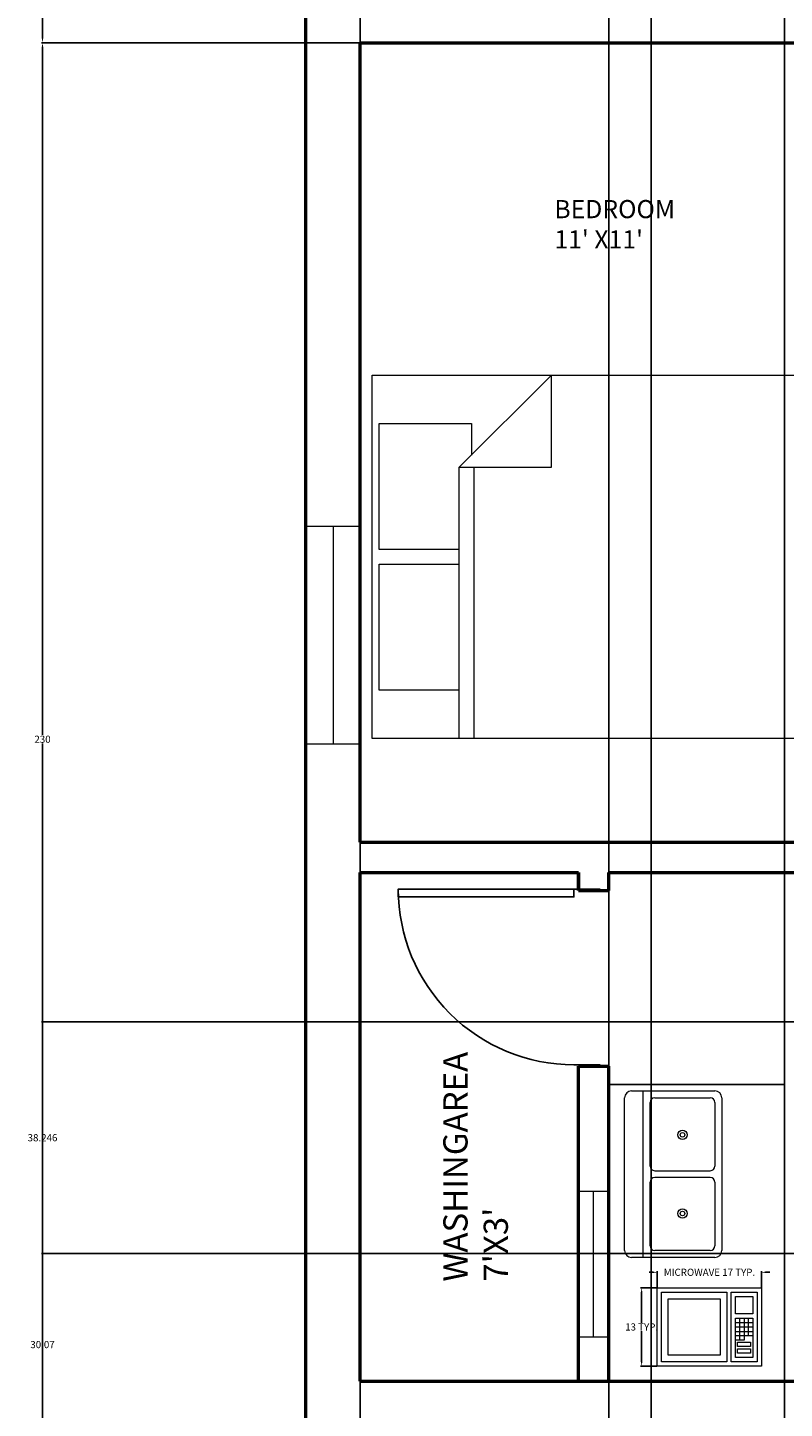
# Model space of a CAD drawing. Units: inches. Extents: x 3506 to 3958, y 1553 to 2506.
# Tile 3 of 16: x 3506 to 3631, y 1775 to 2003. Entities that reach past the tile are written whole.
import ezdxf

# ---------------------------------------------------------------- set-up
doc = ezdxf.new("R2010")
doc.units = ezdxf.units.IN
doc.header["$MEASUREMENT"] = 0
for name, color, linetype, lineweight in [('A-ANNO-DIMS', 2, 'Continuous', 18), ('A-AREA-IDEN', 7, 'Continuous', 18), ('A-FLOR-CASE', 7, 'Continuous', 25), ('A-WALL', 7, 'Continuous', 50), ('doors', 40, 'Continuous', 25), ('furniture', 120, 'Continuous', 18), ('kitchen', 181, 'Continuous', 18), ('window', 30, 'Continuous', 20)]:
    doc.layers.add(name, color=color, linetype=linetype, lineweight=lineweight)
doc.layers.add('A-WALL-PATT', color=251, linetype='Continuous', lineweight=13, true_color=0x636466)
doc.styles.get("Standard").update_dxf_attribs({"font": 'arial.ttf'})
doc.dimstyles.get("Standard").update_dxf_attribs({"dimtxt": 1.18, "dimasz": 0.68, "dimexe": 0.18, "dimexo": 0.0625, "dimgap": 0.09, "dimtad": 0, "dimtih": 1, "dimtoh": 1, "dimdec": 1, "dimzin": 0, "dimdsep": 46, "dimlunit": 3, "dimtxsty": 'Standard', "dimcen": 0.09, "dimadec": 0, "dimazin": 0, "dimtfac": 1, "dimtdec": 1, "dimtofl": 0, "dimtmove": 0, "dimatfit": 3, "dimfxl": 1, "dimtolj": 1, "dimtzin": 0, "dimarcsym": 0})

# ---------------------------------------------------------------- blocks, each defined once
blk = doc.blocks.new('*U12')
for p, q in [((0, 0), (0, 6)), ((40, 0), (40, 6))]:
    blk.add_line(p, q)
blk.add_lwpolyline([(0, 0), (0, -40), (1.75, -40), (1.75, 0)], close=True)
blk.add_arc((0, 0), 40, 270, 0)
blk = doc.blocks.new('Bed - Queen')
for p, q in [((0, -80.00003), (0, 0)), ((0, 0), (59.99999, 0)), ((59.99999, 0), (59.99999, -80.00003)), ((7.99999, -1.2), (28.79998, -1.2)), ((7.99999, -14.4), (7.99999, -1.2)), ((28.79998, -1.2), (28.79998, -14.4)), ((31.19999, -1.2), (51.99999, -1.2)), ((31.19999, -14.4), (31.19999, -1.2)), ((51.99999, -1.2), (51.99999, -16.4)), ((0, -14.4), (44.8, -14.4)), ((59.99999, -29.6), (44.8, -14.4)), ((44.8, -14.4), (44.8, -29.6)), ((44.8, -16.8), (0, -16.8)), ((51.99999, -16.4), (46.79936, -16.4)), ((44.8, -29.6), (59.99999, -29.6)), ((59.99999, -80.00003), (0, -80.00003))]:
    blk.add_line(p, q)
blk = doc.blocks.new('Microwave')
for p, q in [((18, 10), (22, 10)), ((19, 7), (19, 11)), ((20, 11), (20, 7)), ((21, 7), (21, 11)), ((22, 9), (18, 9)), ((18, 8), (22, 8)), ((22, 7), (18, 7)), ((19, 6), (19, 7)), ((20, 7), (20, 6)), ((20, 6), (18, 6))]:
    blk.add_line(p, q)
for points in [[(0, 0), (0, 18), (24, 18), (24, 0)], [(1, 1), (1, 17), (16, 17), (16, 1)], [(17, 1), (17, 17), (23, 17), (23, 1)], [(18, 12), (18, 16), (22, 16), (22, 12)], [(2.5, 2.5), (2.5, 15.5), (14.5, 15.5), (14.5, 2.5)], [(18, 2), (18, 11), (22, 11), (22, 2)], [(18.5, 4.5), (18.5, 5.5), (21.5, 5.5), (21.5, 4.5)], [(18.5, 3), (18.5, 4), (21.5, 4), (21.5, 3)]]:
    blk.add_lwpolyline(points, close=True)
blk = doc.blocks.new('Sink-double - 36 in top')
for p, q in [((-18, -4), (18, -4)), ((-0.75, -18.5), (-0.75, -6.5)), ((0.75, -6.5), (0.75, -18.5))]:
    blk.add_line(p, q)
for points in [[(-16.5, 0), (16.5, 0)], [(-18, -19.5), (-18, -1.5)], [(18, -1.5), (18, -19.5)], [(-15.5, -5.5), (-1.75, -5.5)], [(1.75, -5.5), (15.5, -5.5)], [(-16.5, -18.5), (-16.5, -6.5)], [(16.5, -6.5), (16.5, -18.5)], [(-1.75, -19.5), (-15.5, -19.5)], [(15.5, -19.5), (1.75, -19.5)], [(16.5, -21), (-16.5, -21)]]:
    blk.add_lwpolyline(points)
for centre, radius in [((-8.5, -12.5), 1), ((8.5, -12.5), 1), ((-8.5, -12.5), 0.5), ((8.5, -12.5), 0.5)]:
    blk.add_circle(centre, radius)
for centre, radius, start, end in [((-16.5, -1.5), 1.5, 90, 180), ((16.5, -1.5), 1.5, 0, 90), ((-15.5, -6.5), 1, 90, 180), ((-1.75, -6.5), 1, 0, 90), ((1.75, -6.5), 1, 90, 180), ((15.5, -6.5), 1, 0, 90), ((-16.5, -19.5), 1.5, 180, 270), ((-15.5, -18.5), 1, 180, 270), ((-1.75, -18.5), 1, 270, 0), ((1.75, -18.5), 1, 180, 270), ((15.5, -18.5), 1, 270, 0), ((16.5, -19.5), 1.5, 270, 0)]:
    blk.add_arc(centre, radius, start, end)
blk = doc.blocks.new('WIN-36IN-9IN-WALL')
for p, q in [((0, 9), (0, 0)), ((36, 9), (0, 9)), ((0, 9), (0, 4.5)), ((36, 0), (36, 9)), ((0, 4.5), (36, 4.5)), ((0, 0), (36, 0))]:
    blk.add_line(p, q)
blk = doc.blocks.new('WIN-24IN-5IN-PARTITION')
for p, q in [((5, 24), (0, 24)), ((0, 24), (0, 0)), ((2.5, 0), (2.5, 24)), ((5, 0), (5, 24)), ((0, 0), (5, 0)), ((0, 0), (2.5, 0))]:
    blk.add_line(p, q)
blk = doc.blocks.new('*D20')
at = {"layer": 'A-ANNO-DIMS', "color": 0, "lineweight": -2, "transparency": 16777216}
for p, q in [((3609.07, 1797.37), (3608.39, 1797.37)), ((3609.75, 1794.85), (3609.75, 1797.55)), ((3626.96, 1794.85), (3626.96, 1797.55)), ((3627.64, 1797.37), (3628.32, 1797.37))]:
    blk.add_line(p, q, dxfattribs=at)
at = {"layer": 'A-ANNO-DIMS', "color": 0, "transparency": 16777216}
for points in [[(3609.07, 1797.48), (3609.07, 1797.25), (3609.75, 1797.37)], [(3627.64, 1797.48), (3627.64, 1797.25), (3626.96, 1797.37)]]:
    blk.add_solid(points, dxfattribs=at)
at = {"layer": 'Defpoints', "color": 0, "transparency": 16777216}
for p in [(3626.96, 1797.37), (3609.75, 1794.79), (3626.96, 1794.79)]:
    blk.add_point(p, dxfattribs=at)
at = {"layer": 'A-ANNO-DIMS', "color": 0, "transparency": 16777216, "insert": (3618.36, 1797.37), "char_height": 1.18, "attachment_point": 5}
blk.add_mtext('\\A1;MICROWAVE 17 TYP.', dxfattribs=at)
blk = doc.blocks.new('*D21')
at = {"layer": 'A-ANNO-DIMS', "color": 0, "lineweight": -2, "transparency": 16777216}
for p, q in [((3609.69, 1794.79), (3606.99, 1794.79)), ((3607.17, 1794.11), (3607.17, 1789.03)), ((3607.17, 1782.56), (3607.17, 1787.64)), ((3609.69, 1781.88), (3606.99, 1781.88))]:
    blk.add_line(p, q, dxfattribs=at)
at = {"layer": 'A-ANNO-DIMS', "color": 0, "transparency": 16777216}
for points in [[(3607.06, 1794.11), (3607.29, 1794.11), (3607.17, 1794.79)], [(3607.06, 1782.56), (3607.29, 1782.56), (3607.17, 1781.88)]]:
    blk.add_solid(points, dxfattribs=at)
at = {"layer": 'Defpoints', "color": 0, "transparency": 16777216}
for p in [(3607.17, 1794.79), (3609.75, 1794.79), (3609.75, 1781.88)]:
    blk.add_point(p, dxfattribs=at)
at = {"layer": 'A-ANNO-DIMS', "color": 0, "transparency": 16777216, "insert": (3607.17, 1788.34), "char_height": 1.18, "attachment_point": 5}
blk.add_mtext('\\A1;13 TYP.', dxfattribs=at)
blk = doc.blocks.new('*D42')
at = {"layer": 'A-ANNO-DIMS', "color": 0, "lineweight": -2, "transparency": 16777216}
for p, q in [((3560.67, 2000.39), (3508.1, 2000.39)), ((3508.28, 1999.71), (3508.28, 1886.09)), ((3508.28, 1771.07), (3508.28, 1884.7)), ((3560.67, 1770.39), (3508.1, 1770.39))]:
    blk.add_line(p, q, dxfattribs=at)
at = {"layer": 'A-ANNO-DIMS', "color": 0, "transparency": 16777216}
for points in [[(3508.17, 1999.71), (3508.39, 1999.71), (3508.28, 2000.39)], [(3508.17, 1771.07), (3508.39, 1771.07), (3508.28, 1770.39)]]:
    blk.add_solid(points, dxfattribs=at)
at = {"layer": 'Defpoints', "color": 0, "transparency": 16777216}
for p in [(3508.28, 2000.39), (3560.73, 2000.39), (3560.73, 1770.39)]:
    blk.add_point(p, dxfattribs=at)
at = {"layer": 'A-ANNO-DIMS', "color": 0, "transparency": 16777216, "insert": (3508.28, 1885.39), "char_height": 1.18, "attachment_point": 5}
blk.add_mtext('\\A1;230', dxfattribs=at)
blk = doc.blocks.new('*D43')
at = {"layer": 'A-ANNO-DIMS', "color": 0, "lineweight": -2, "transparency": 16777216}
for p, q in [((3560.67, 2226.39), (3508.1, 2226.39)), ((3508.28, 2225.71), (3508.28, 2114.09)), ((3508.28, 2001.07), (3508.28, 2112.7)), ((3560.67, 2000.39), (3508.1, 2000.39))]:
    blk.add_line(p, q, dxfattribs=at)
at = {"layer": 'A-ANNO-DIMS', "color": 0, "transparency": 16777216}
for points in [[(3508.17, 2225.71), (3508.39, 2225.71), (3508.28, 2226.39)], [(3508.17, 2001.07), (3508.39, 2001.07), (3508.28, 2000.39)]]:
    blk.add_solid(points, dxfattribs=at)
at = {"layer": 'Defpoints', "color": 0, "transparency": 16777216}
for p in [(3508.28, 2226.39), (3560.73, 2226.39), (3560.73, 2000.39)]:
    blk.add_point(p, dxfattribs=at)
at = {"layer": 'A-ANNO-DIMS', "color": 0, "transparency": 16777216, "insert": (3508.28, 2113.39), "char_height": 1.18, "attachment_point": 5}
blk.add_mtext('\\A1;226', dxfattribs=at)
blk = doc.blocks.new('*D50')
at = {"layer": 'A-ANNO-DIMS', "color": 0, "lineweight": -2, "transparency": 16777216}
for p, q in [((3608.73, 1606.46), (3608.73, 2505.02)), ((3609.41, 2504.84), (3672.39, 2504.84)), ((3738.05, 2504.84), (3675.07, 2504.84)), ((3738.73, 1606.46), (3738.73, 2505.02))]:
    blk.add_line(p, q, dxfattribs=at)
at = {"layer": 'A-ANNO-DIMS', "color": 0, "transparency": 16777216}
for points in [[(3609.41, 2504.96), (3609.41, 2504.73), (3608.73, 2504.84)], [(3738.05, 2504.96), (3738.05, 2504.73), (3738.73, 2504.84)]]:
    blk.add_solid(points, dxfattribs=at)
at = {"layer": 'Defpoints', "color": 0, "transparency": 16777216}
for p in [(3738.73, 2504.84), (3608.73, 1606.39), (3738.73, 1606.39)]:
    blk.add_point(p, dxfattribs=at)
at = {"layer": 'A-ANNO-DIMS', "color": 0, "transparency": 16777216, "insert": (3673.73, 2504.84), "char_height": 1.18, "attachment_point": 5}
blk.add_mtext('\\A1;130', dxfattribs=at)
blk = doc.blocks.new('*D52')
at = {"layer": 'A-ANNO-DIMS', "color": 0, "lineweight": -2, "transparency": 16777216}
for p, q in [((3560.73, 1606.46), (3560.73, 2505.02)), ((3561.41, 2504.84), (3583.77, 2504.84)), ((3608.05, 2504.84), (3585.69, 2504.84)), ((3608.73, 1606.46), (3608.73, 2505.02))]:
    blk.add_line(p, q, dxfattribs=at)
at = {"layer": 'A-ANNO-DIMS', "color": 0, "transparency": 16777216}
for points in [[(3561.41, 2504.96), (3561.41, 2504.73), (3560.73, 2504.84)], [(3608.05, 2504.96), (3608.05, 2504.73), (3608.73, 2504.84)]]:
    blk.add_solid(points, dxfattribs=at)
at = {"layer": 'Defpoints', "color": 0, "transparency": 16777216}
for p in [(3608.73, 2504.84), (3560.73, 1606.39), (3608.73, 1606.39)]:
    blk.add_point(p, dxfattribs=at)
at = {"layer": 'A-ANNO-DIMS', "color": 0, "transparency": 16777216, "insert": (3584.73, 2504.84), "char_height": 1.18, "attachment_point": 5}
blk.add_mtext('\\A1;48', dxfattribs=at)
blk = doc.blocks.new('*D62')
at = {"layer": 'A-ANNO-DIMS', "color": 0, "lineweight": -2, "transparency": 16777216}
for p, q in [((3860.67, 1838.71), (3508.1, 1838.71)), ((3508.28, 1838.03), (3508.28, 1820.28)), ((3508.28, 1801.14), (3508.28, 1818.89)), ((3860.67, 1800.46), (3508.1, 1800.46))]:
    blk.add_line(p, q, dxfattribs=at)
at = {"layer": 'A-ANNO-DIMS', "color": 0, "transparency": 16777216}
for points in [[(3508.17, 1838.03), (3508.39, 1838.03), (3508.28, 1838.71)], [(3508.17, 1801.14), (3508.39, 1801.14), (3508.28, 1800.46)]]:
    blk.add_solid(points, dxfattribs=at)
at = {"layer": 'Defpoints', "color": 0, "transparency": 16777216}
for p in [(3860.73, 1838.71), (3508.28, 1800.46), (3860.73, 1800.46)]:
    blk.add_point(p, dxfattribs=at)
at = {"layer": 'A-ANNO-DIMS', "color": 0, "transparency": 16777216, "insert": (3508.28, 1819.59), "char_height": 1.18, "attachment_point": 5}
blk.add_mtext('\\A1;38.246', dxfattribs=at)
blk = doc.blocks.new('*D63')
at = {"layer": 'A-ANNO-DIMS', "color": 0, "lineweight": -2, "transparency": 16777216}
for p, q in [((3869.67, 1800.46), (3508.1, 1800.46)), ((3508.28, 1799.78), (3508.28, 1786.12)), ((3508.28, 1771.07), (3508.28, 1784.74)), ((3869.67, 1770.39), (3508.1, 1770.39))]:
    blk.add_line(p, q, dxfattribs=at)
at = {"layer": 'A-ANNO-DIMS', "color": 0, "transparency": 16777216}
for points in [[(3508.17, 1799.78), (3508.39, 1799.78), (3508.28, 1800.46)], [(3508.17, 1771.07), (3508.39, 1771.07), (3508.28, 1770.39)]]:
    blk.add_solid(points, dxfattribs=at)
at = {"layer": 'Defpoints', "color": 0, "transparency": 16777216}
for p in [(3869.73, 1800.46), (3508.28, 1770.39), (3869.73, 1770.39)]:
    blk.add_point(p, dxfattribs=at)
at = {"layer": 'A-ANNO-DIMS', "color": 0, "transparency": 16777216, "insert": (3508.28, 1785.43), "char_height": 1.18, "attachment_point": 5}
blk.add_mtext('\\A1;30.07', dxfattribs=at)
blk = doc.blocks.new('*D68')
at = {"layer": 'A-ANNO-DIMS', "color": 0, "lineweight": -2, "transparency": 16777216}
for p, q in [((3630.73, 2260.33), (3630.73, 1553.76)), ((3601.73, 2231.33), (3601.73, 1553.76)), ((3602.41, 1553.94), (3615.28, 1553.94)), ((3630.05, 1553.94), (3617.18, 1553.94))]:
    blk.add_line(p, q, dxfattribs=at)
at = {"layer": 'A-ANNO-DIMS', "color": 0, "transparency": 16777216}
for points in [[(3602.41, 1554.06), (3602.41, 1553.83), (3601.73, 1553.94)], [(3630.05, 1554.06), (3630.05, 1553.83), (3630.73, 1553.94)]]:
    blk.add_solid(points, dxfattribs=at)
at = {"layer": 'Defpoints', "color": 0, "transparency": 16777216}
for p in [(3630.73, 2260.39), (3601.73, 2231.39), (3630.73, 1553.94)]:
    blk.add_point(p, dxfattribs=at)
at = {"layer": 'A-ANNO-DIMS', "color": 0, "transparency": 16777216, "insert": (3616.23, 1553.94), "char_height": 1.18, "attachment_point": 5}
blk.add_mtext('\\A1;29', dxfattribs=at)

msp = doc.modelspace()

# ---------------------------------------------------------------- hatches: boundary and pattern name
at = {"layer": 'A-WALL-PATT'}
h = msp.add_hatch(dxfattribs=at)
h.set_pattern_fill('ANSI31', color=256)
h.paths.add_polyline_path([(3911.7302, 2461.3942), (3551.7302, 2461.3942), (3551.7302, 2152.516), (3560.7302, 2152.516), (3560.7302, 2116.516), (3551.7302, 2116.516), (3551.7302, 1920.5711), (3556.2302, 1920.5711), (3560.7302, 1920.5711), (3560.7302, 2000.3942), (3692.7302, 2000.3942), (3692.7302, 1997.3942), (3697.7302, 1997.3942), (3697.7302, 2000.3942), (3771.7302, 2000.3942), (3771.7302, 1997.3942), (3776.7302, 1997.3942), (3776.7302, 1997.7206), (3778.5802, 1997.7206), (3807.5802, 1997.7206), (3807.5802, 1996.4519), (3778.5802, 1996.4519), (3778.5802, 1997.7206), (3776.7302, 1997.7206), (3776.7302, 1997.3942), (3771.7302, 1997.3942), (3771.7302, 2000.3942), (3697.7302, 2000.3942), (3697.7302, 1997.3942), (3692.7302, 1997.3942), (3689.8302, 1997.3942), (3689.8302, 1995.8192), (3653.8302, 1995.8192), (3653.8302, 1997.3942), (3689.8302, 1997.3942), (3692.7302, 1997.3942), (3692.7302, 2000.3942), (3560.7302, 2000.3942), (3560.7302, 1920.5711), (3551.7302, 1920.5711), (3551.7302, 1884.5711), (3551.7302, 1597.3942), (3911.7302, 1597.3942)], flags=17)
h.paths.add_polyline_path([(3596.7302, 2005.3942), (3596.7302, 2057.3035, -0.38730371), (3569.1778, 2085), (3569.15, 2085), (3569.15, 2086.2688), (3598.15, 2086.2688), (3598.15, 2085), (3569.1778, 2085, 0.38730371), (3596.7302, 2057.3035), (3596.7302, 2057.3942), (3601.7302, 2057.3942), (3601.7302, 2055.3942), (3630.7302, 2055.3942), (3630.7302, 2034.3942), (3694.7302, 2034.3942), (3694.7302, 2053.3942), (3699.7302, 2053.3942), (3699.7302, 2005.3942), (3860.7302, 2005.3942), (3860.7302, 2173.3942), (3771.7302, 2173.3942), (3771.7302, 2194.3942), (3776.7302, 2194.3942), (3776.7302, 2178.3942), (3860.7302, 2178.3942), (3860.7302, 2231.3942), (3601.7302, 2231.3942), (3601.7302, 2241.426), (3596.7302, 2241.426), (3596.7302, 2231.3942), (3560.7302, 2231.3942), (3560.7302, 2315.3942), (3596.7302, 2315.3942), (3596.7302, 2312.3942), (3601.7302, 2312.3942), (3601.7302, 2315.3942), (3697.7302, 2315.3942), (3697.7302, 2413.3942), (3692.7302, 2413.3942), (3692.7302, 2320.3942), (3560.7302, 2320.3942), (3560.7302, 2452.3942), (3692.7302, 2452.3942), (3692.7302, 2449.3942), (3697.7302, 2449.3942), (3697.7302, 2452.3942), (3771.7302, 2452.3942), (3771.7302, 2449.3942), (3776.7302, 2449.3942), (3776.7302, 2452.3942), (3860.7302, 2452.3942), (3860.7302, 2437.2075), (3865.2302, 2437.2075), (3865.2302, 2413.2075), (3860.7302, 2413.2075), (3860.7302, 2367.6976), (3865.2302, 2367.6976), (3869.7302, 2367.6976), (3869.7302, 2319.6976), (3860.7302, 2319.6976), (3860.7302, 2211.6248), (3869.7302, 2211.6248), (3869.7302, 2187.6248), (3860.7302, 2187.6248), (3860.7302, 2138.4346), (3865.2302, 2138.4346), (3869.7302, 2138.4346), (3869.7302, 2090.4346), (3860.7302, 2090.4346), (3860.7302, 1985.8449), (3869.7302, 1985.8449), (3869.7302, 1961.8449), (3860.7302, 1961.8449), (3860.7302, 1897.0756), (3865.2302, 1897.0756), (3869.7302, 1897.0756), (3869.7302, 1849.0756), (3860.7302, 1849.0756), (3860.7302, 1847.8112), (3860.7302, 1779.3942), (3596.7302, 1779.3942), (3596.7302, 1831.3942), (3601.7302, 1831.3942), (3601.7302, 1828.3942), (3630.7302, 1828.3942), (3630.7302, 1808.3942), (3691.7302, 1808.3942), (3691.7302, 1815.3942), (3696.7302, 1815.3942), (3696.7302, 1779.3942), (3860.7302, 1779.3942), (3860.7302, 1947.3942), (3771.7302, 1947.3942), (3771.7302, 1968.3942), (3776.7302, 1968.3942), (3776.7302, 1952.3942), (3860.7302, 1952.3942), (3860.7302, 2005.3942)], flags=0)
h.paths.add_polyline_path([(3596.7302, 2038.8546), (3601.7302, 2038.8546), (3601.7302, 2014.8546), (3596.7302, 2014.8546)], flags=0)
h.paths.add_polyline_path([(3564.1688, 2107), (3564.1688, 2167), (3644.1688, 2167), (3644.1688, 2107)], flags=0)
h.paths.add_polyline_path([(3607.0972, 2052.0208), (3620.8472, 2052.0208, -0.41421356), (3621.9931, 2050.875), (3621.9931, 2025.6667, -0.41421356), (3620.8472, 2024.5208), (3607.0972, 2024.5208, -0.41421356), (3605.9514, 2025.6667), (3605.9514, 2050.875, -0.41421356)], flags=0)
h.paths.add_polyline_path([(3578.5688, 2115), (3565.3688, 2115), (3565.3688, 2135.8), (3578.5688, 2135.8), (3578.5688, 2138.2), (3565.3688, 2138.2), (3565.3688, 2159), (3580.5688, 2159), (3580.5688, 2153.8), (3593.7688, 2167), (3593.7688, 2151.8), (3578.5688, 2151.8)], flags=0)
h.paths.add_polyline_path([(3610.9167, 2050.875), (3620.0833, 2050.875, -0.41421356), (3620.8472, 2050.1111), (3620.8472, 2039.6076, -0.41421356), (3620.0833, 2038.8438), (3610.9167, 2038.8438, -0.41421356), (3610.1528, 2039.6076), (3610.1528, 2050.1111, -0.41421356)], flags=0)
h.paths.add_polyline_path([(3610.9167, 2037.6979), (3620.0833, 2037.6979, -0.41421356), (3620.8472, 2036.934), (3620.8472, 2026.4306, -0.41421356), (3620.0833, 2025.6667), (3610.9167, 2025.6667, -0.41421356), (3610.1528, 2026.4306), (3610.1528, 2036.934, -0.41421356)], flags=0)
h.paths.add_polyline_path([(3616.2639, 2044.7639, -1), (3614.7361, 2044.7639, -1)], flags=0)
h.paths.add_polyline_path([(3615.8819, 2044.7639, -1), (3615.1181, 2044.7639, -1)], flags=0)
h.paths.add_polyline_path([(3616.2639, 2031.7778, -1), (3614.7361, 2031.7778, -1)], flags=0)
h.paths.add_polyline_path([(3615.8819, 2031.7778, -1), (3615.1181, 2031.7778, -1)], flags=0)
h.paths.add_polyline_path([(3609.7539, 2021.7868), (3626.9586, 2021.7868), (3626.9586, 2008.8833), (3609.7539, 2008.8833)], flags=0)
h.paths.add_polyline_path([(3610.4708, 2021.07), (3621.2237, 2021.07), (3621.2237, 2009.6002), (3610.4708, 2009.6002)], flags=0)
h.paths.add_polyline_path([(3611.5461, 2019.9947), (3620.1484, 2019.9947), (3620.1484, 2010.6755), (3611.5461, 2010.6755)], flags=0)
h.paths.add_polyline_path([(3621.9405, 2021.07), (3626.2417, 2021.07), (3626.2417, 2009.6002), (3621.9405, 2009.6002)], flags=0)
h.paths.add_polyline_path([(3622.6574, 2020.3531), (3625.5248, 2020.3531), (3625.5248, 2017.4857), (3622.6574, 2017.4857)], flags=0)
h.paths.add_polyline_path([(3622.6574, 2016.7688), (3625.5248, 2016.7688), (3625.5248, 2010.317), (3622.6574, 2010.317)], flags=0)
h.paths.add_polyline_path([(3624.808, 2016.0519), (3624.808, 2013.9013), (3624.0911, 2013.9013), (3624.0911, 2013.1845), (3623.3743, 2013.1845), (3623.3743, 2013.9013), (3623.3743, 2016.0519)], flags=0)
h.paths.add_polyline_path([(3623.0158, 2012.8261), (3625.1664, 2012.8261), (3625.1664, 2012.1092), (3623.0158, 2012.1092)], flags=0)
h.paths.add_polyline_path([(3623.0158, 2011.7508), (3625.1664, 2011.7508), (3625.1664, 2011.0339), (3623.0158, 2011.0339)], flags=0)
h.paths.add_polyline_path([(3650.0591, 2031.8202), (3674.0368, 2031.8202), (3674.0368, 2012.638), (3669.2413, 2012.638), (3669.2413, 2011.8388), (3672.4383, 2011.8388), (3672.4383, 2011.0395), (3651.6576, 2011.0395), (3651.6576, 2011.8388), (3654.8546, 2011.8388), (3654.8546, 2012.638), (3650.0591, 2012.638)], flags=0)
h.paths.add_polyline_path([(3658.0517, 2024.6269, -1), (3651.6576, 2024.6269, -1)], flags=0)
h.paths.add_polyline_path([(3657.2524, 2024.6269, -1), (3652.4569, 2024.6269, -1)], flags=0)
h.paths.add_polyline_path([(3656.4532, 2024.6269, -1), (3653.2561, 2024.6269, -1)], flags=0)
h.paths.add_polyline_path([(3655.6539, 2024.6269, -1), (3654.0554, 2024.6269, -1)], flags=0)
h.paths.add_polyline_path([(3657.2524, 2017.4336, -1), (3652.4569, 2017.4336, -1)], flags=0)
h.paths.add_polyline_path([(3656.4532, 2017.4336, -1), (3653.2561, 2017.4336, -1)], flags=0)
h.paths.add_polyline_path([(3655.6539, 2017.4336, -1), (3654.0554, 2017.4336, -1)], flags=0)
h.paths.add_polyline_path([(3659.6502, 2027.8239), (3664.4457, 2027.8239), (3664.4457, 2015.0358), (3659.6502, 2015.0358)], flags=0)
h.paths.add_polyline_path([(3663.6465, 2027.0247), (3663.6465, 2015.8351), (3660.4494, 2015.8351), (3660.4494, 2027.0247)], flags=0)
h.paths.add_polyline_path([(3562.6688, 1945.5), (3642.6688, 1945.5), (3642.6688, 1885.5), (3562.6688, 1885.5)], flags=0)
h.paths.add_polyline_path([(3671.6391, 2024.6269, -1), (3666.8435, 2024.6269, -1)], flags=0)
h.paths.add_polyline_path([(3670.8398, 2024.6269, -1), (3667.6428, 2024.6269, -1)], flags=0)
h.paths.add_polyline_path([(3672.4383, 2017.4336, -1), (3666.0443, 2017.4336, -1)], flags=0)
h.paths.add_polyline_path([(3670.0405, 2024.6269, -1), (3668.442, 2024.6269, -1)], flags=0)
h.paths.add_polyline_path([(3671.6391, 2017.4336, -1), (3666.8435, 2017.4336, -1)], flags=0)
h.paths.add_polyline_path([(3670.8398, 2017.4336, -1), (3667.6428, 2017.4336, -1)], flags=0)
h.paths.add_polyline_path([(3592.2688, 1945.5), (3592.2688, 1930.3), (3577.0688, 1930.3), (3577.0688, 1893.5), (3563.8688, 1893.5), (3563.8688, 1914.3), (3577.0688, 1914.3), (3577.0688, 1916.7), (3563.8688, 1916.7), (3563.8688, 1937.5), (3579.0688, 1937.5), (3579.0688, 1932.3)], flags=0)
h.paths.add_polyline_path([(3670.0405, 2017.4336, -1), (3668.442, 2017.4336, -1)], flags=0)
h.paths.add_polyline_path([(3596.7302, 2283.3942), (3601.7302, 2283.3942), (3601.7302, 2265.426), (3599.2302, 2265.426), (3599.2302, 2241.426), (3596.7302, 2241.426), (3596.7302, 2265.426)], flags=0)
h.paths.add_polyline_path([(3596.7302, 1810.7006), (3601.7302, 1810.7006), (3601.7302, 1786.7006), (3596.7302, 1786.7006)], flags=0)
h.paths.add_polyline_path([(3560.7302, 1770.3942), (3738.7302, 1770.3942), (3738.7302, 1746.3942), (3738.7302, 1722.3942), (3748.7302, 1722.3942), (3748.7302, 1674.3942), (3560.7302, 1674.3942)], flags=0)
h.paths.add_polyline_path([(3728.7302, 1746.3942), (3728.7302, 1756.0642), (3738.7302, 1746.3942), (3728.7302, 1738.1582), (3728.7302, 1698.3942), (3591.2519, 1698.3942), (3591.2519, 1746.3942)], flags=0)
h.paths.add_polyline_path([(3771.7302, 2399.3942), (3771.7302, 2420.3942), (3776.7302, 2420.3942), (3776.7302, 2404.3942), (3776.7302, 2399.3942)], flags=0)
h.paths.add_polyline_path([(3911.7302, 2461.3942), (3551.7302, 2461.3942), (3551.7302, 2152.516), (3560.7302, 2152.516), (3560.7302, 2116.516), (3551.7302, 2116.516), (3551.7302, 1920.5711), (3560.7302, 1920.5711), (3560.7302, 2000.3942), (3692.7302, 2000.3942), (3692.7302, 1997.3942), (3697.7302, 1997.3942), (3697.7302, 2000.3942), (3771.7302, 2000.3942), (3771.7302, 1997.3942), (3776.7302, 1997.3942), (3776.7302, 1997.7206), (3778.5802, 1997.7206), (3807.5802, 1997.7206), (3807.5802, 1996.4519), (3778.5802, 1996.4519), (3778.5802, 1997.7206), (3776.7302, 1997.7206), (3776.7302, 1997.3942), (3771.7302, 1997.3942), (3771.7302, 2000.3942), (3697.7302, 2000.3942), (3697.7302, 1997.3942), (3692.7302, 1997.3942), (3689.8302, 1997.3942), (3689.8302, 1995.8192), (3653.8302, 1995.8192), (3653.8302, 1997.3942), (3689.8302, 1997.3942), (3692.7302, 1997.3942), (3692.7302, 2000.3942), (3560.7302, 2000.3942), (3560.7302, 1920.5711), (3551.7302, 1920.5711), (3551.7302, 1597.3942), (3911.7302, 1597.3942)], flags=17)

# ---------------------------------------------------------------- linework, layer by layer
at = {"layer": 'A-FLOR-CASE'}
msp.add_line((3601.7302, 1828.3942), (3630.7302, 1828.3942), dxfattribs=at)
at = {"layer": 'A-WALL'}
for p, q in [((3560.7302, 2000.3942), (3692.7302, 2000.3942)), ((3560.7302, 1868.3942), (3560.7302, 2000.3942)), ((3560.7302, 1868.3942), (3692.7302, 1868.3942)), ((3560.7302, 1863.3942), (3596.7302, 1863.3942)), ((3560.7302, 1779.3942), (3560.7302, 1863.3942)), ((3596.7302, 1863.3942), (3596.7302, 1860.3942)), ((3596.7302, 1860.3942), (3596.7302, 1863.3942)), ((3601.7302, 1863.3942), (3697.7302, 1863.3942)), ((3601.7302, 1860.3942), (3601.7302, 1863.3942)), ((3596.7302, 1860.3942), (3601.7302, 1860.3942)), ((3596.7302, 1779.3942), (3596.7302, 1831.3942)), ((3596.7302, 1831.3942), (3601.7302, 1831.3942)), ((3601.7302, 1779.3942), (3601.7302, 1831.3942)), ((3560.7302, 1779.3942), (3771.7302, 1779.3942))]:
    msp.add_line(p, q, dxfattribs=at)
msp.add_lwpolyline([(3551.7302, 2461.3942), (3911.7302, 2461.3942), (3911.7302, 1597.3942), (3551.7302, 1597.3942)], close=True, dxfattribs=at)

# ---------------------------------------------------------------- block references
at = {"layer": 'doors', "xscale": 0.725, "yscale": 0.725, "zscale": 0.725, "rotation": 270}
msp.add_blockref('*U12', (3596, 1860.6344), dxfattribs=at)
at = {"layer": 'furniture', "rotation": 90}
msp.add_blockref('Bed - Queen', (3562.6688, 1885.5), dxfattribs=at)
at = {"layer": 'kitchen', "xscale": 0.763888888888889, "yscale": 0.763888888888889, "zscale": 0.763888888888889, "rotation": 90}
msp.add_blockref('Sink-double - 36 in top', (3604.3681, 1813.5729), dxfattribs=at)
at = {"layer": 'kitchen', "xscale": 0.7168604389202189, "yscale": 0.7168604389202189, "zscale": 0.7168604389202189}
msp.add_blockref('Microwave', (3609.7539, 1781.8833), dxfattribs=at)
at = {"layer": 'window', "extrusion": (0, 0, -1), "zscale": -1, "rotation": 269.9999999999985}
msp.add_blockref('WIN-36IN-9IN-WALL', (-3560.7304, 1920.571), dxfattribs=at)
at = {"layer": 'window'}
msp.add_blockref('WIN-24IN-5IN-PARTITION', (3596.73, 1786.701), dxfattribs=at)

# ---------------------------------------------------------------- texts
at = {"layer": 'A-AREA-IDEN', "insert": (3592.7677, 1974.4257), "char_height": 3, "attachment_point": 1}
msp.add_mtext_dynamic_manual_height_columns("BEDROOM\\P11' X11'", width=46.119714, gutter_width=1, heights=[0], dxfattribs=at)
at = {"layer": 'A-AREA-IDEN', "insert": (3574.4345, 1795.8246), "char_height": 4, "attachment_point": 1, "rotation": 90}
msp.add_mtext_dynamic_manual_height_columns("WASHINGAREA\\P 7'X3'", width=7.450055, gutter_width=1, heights=[0], dxfattribs=at)

# ---------------------------------------------------------------- dimensions: what is measured, and where the dimension line sits
at = {"layer": 'A-ANNO-DIMS'}
for base, p1, p2, picture, middle in [((3608.7302, 2504.8442), (3560.7302, 1606.3942), (3608.7302, 1606.3942), '*D52', (3584.7302, 2504.8442)), ((3738.7302, 2504.8442), (3608.7302, 1606.3942), (3738.7302, 1606.3942), '*D50', (3673.7302, 2504.8442)), ((3630.7302, 1553.9442), (3601.7302, 2231.3942), (3630.7302, 2260.3942), '*D68', (3616.2302, 1553.9442))]:
    dim = msp.add_linear_dim(base=base, p1=p1, p2=p2, dimstyle='Standard', override={"dimdec": 0, "dimlfac": 1, "dimrnd": 0, "dimzin": 0, "dimdsep": 46, "dimlunit": 2}, dxfattribs=at)
    dim.commit()
    dim.dimension.update_dxf_attribs({"geometry": picture, "text_midpoint": middle})
for base, p1, p2, override, picture, middle in [((3508.2802, 2226.3942), (3560.7302, 2000.3942), (3560.7302, 2226.3942), {"dimdec": 0, "dimlfac": 1, "dimrnd": 0, "dimzin": 0, "dimdsep": 46, "dimlunit": 2}, '*D43', (3508.2802, 2113.3942)), ((3508.2802, 2000.3942), (3560.7302, 1770.3942), (3560.7302, 2000.3942), {"dimdec": 0, "dimlfac": 1, "dimrnd": 0, "dimzin": 0, "dimdsep": 46, "dimlunit": 2}, '*D42', (3508.2802, 1885.3942)), ((3508.2802, 1800.4628), (3860.7302, 1838.7087), (3860.7302, 1800.4628), {"dimdec": 3, "dimlfac": 1, "dimrnd": 0, "dimzin": 0, "dimdsep": 46, "dimlunit": 2}, '*D62', (3508.2802, 1819.5857)), ((3508.2802, 1770.3942), (3869.7302, 1800.4628), (3869.7302, 1770.3942), {"dimdec": 2, "dimlfac": 1, "dimrnd": 0, "dimzin": 0, "dimdsep": 46, "dimlunit": 2}, '*D63', (3508.2802, 1785.4285))]:
    dim = msp.add_linear_dim(base=base, p1=p1, p2=p2, angle=90, dimstyle='Standard', override=override, dxfattribs=at)
    dim.commit()
    dim.dimension.update_dxf_attribs({"geometry": picture, "text_midpoint": middle})
dim = msp.add_linear_dim(base=(3626.9586, 1797.3675), p1=(3609.7539, 1794.7868), p2=(3626.9586, 1794.7868), text='MICROWAVE <> TYP.', dimstyle='Standard', override={"dimdec": 0, "dimlfac": 1, "dimrnd": 0, "dimzin": 0, "dimdsep": 46, "dimlunit": 2}, dxfattribs=at)
dim.commit()
dim.dimension.update_dxf_attribs({"geometry": '*D20', "text_midpoint": (3618.3562, 1797.3675)})
dim = msp.add_linear_dim(base=(3607.1732, 1794.7868), p1=(3609.7539, 1781.8833), p2=(3609.7539, 1794.7868), angle=90, text='<> TYP.', dimstyle='Standard', override={"dimdec": 0, "dimlfac": 1, "dimrnd": 0, "dimzin": 0, "dimdsep": 46, "dimlunit": 2}, dxfattribs=at)
dim.commit()
dim.dimension.update_dxf_attribs({"geometry": '*D21', "text_midpoint": (3607.1732, 1788.3351)})

doc.saveas('drawing.dxf')
